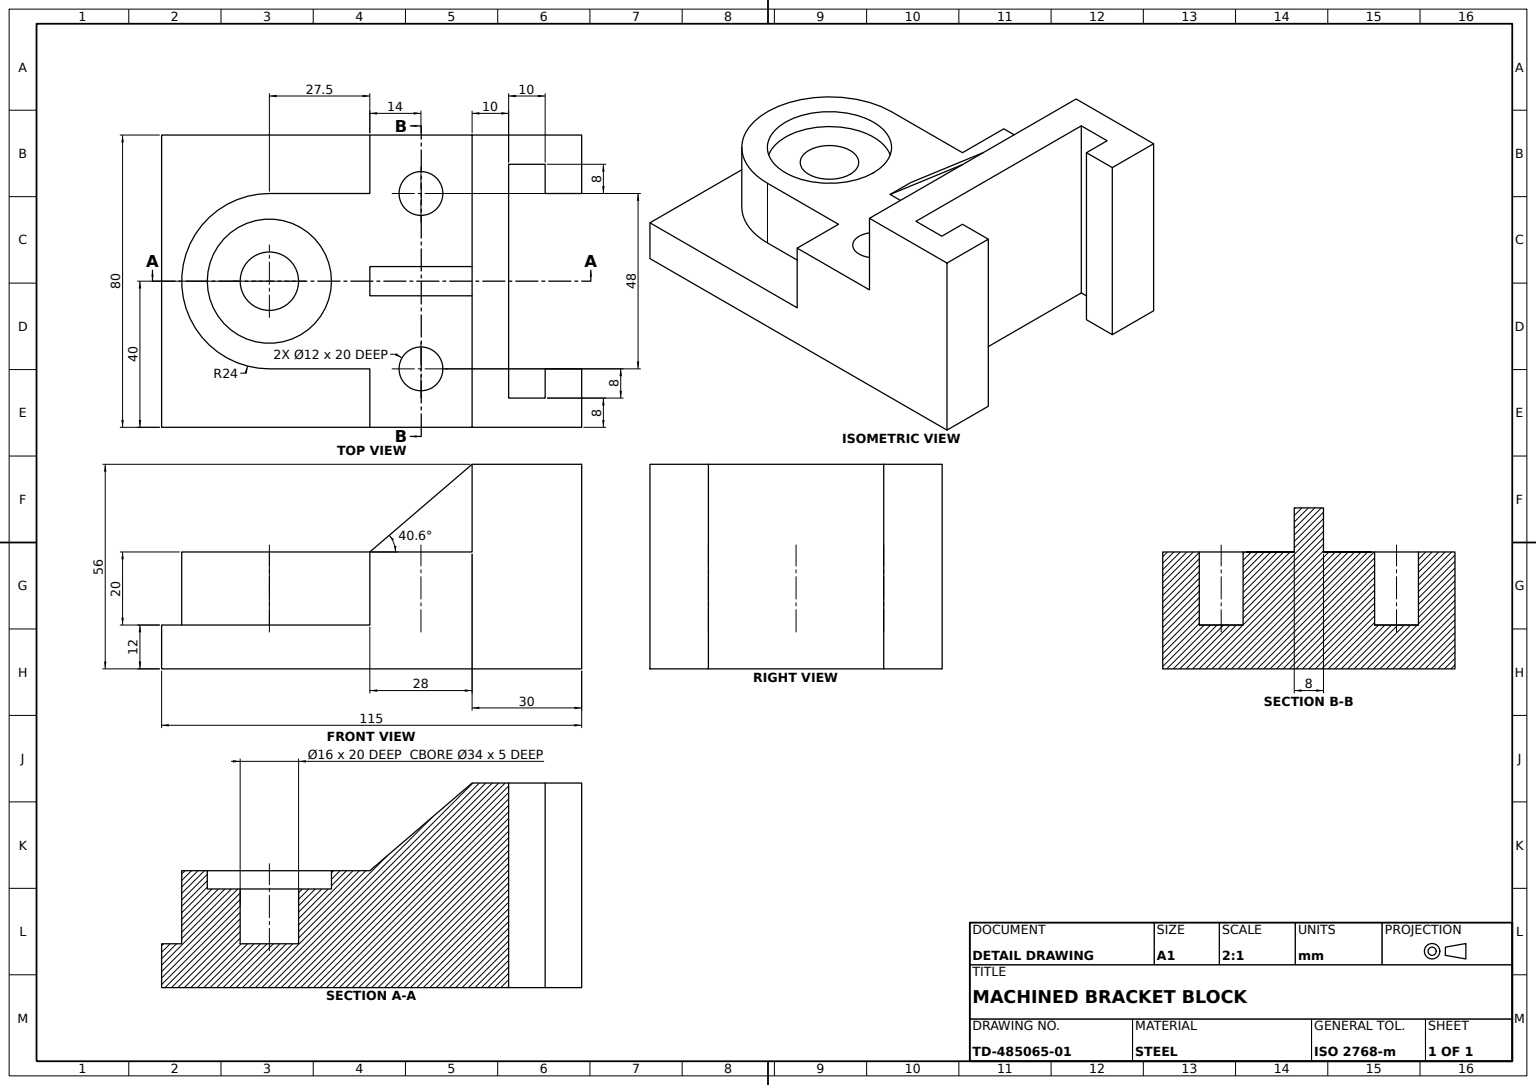
from build123d import *

# Parameters (mm, degrees)
BASE_PLATE_SKETCH_W    = 80
BASE_PLATE_SKETCH_H    = 115
BASE_PLATE_DEPTH       = 12
BACK_WALL_SKETCH_W     = 80
BACK_WALL_SKETCH_H     = 30
BACK_WALL_DEPTH        = 44
WALL_SLOT_CUT_DEPTH    = 90.678592763
BOSS_PAD_SKETCH_R      = 6
BOSS_PAD_DEPTH         = 20
COUNTERBORE_SKETCH_R   = 17
COUNTERBORE_34X5_DEPTH = 5
BORE_SKETCH_R          = 8
BORE_16_DEPTH          = 15
SUPPORT_RIB_8MM_REACH  = 91.679
RIB_SKETCH_WALL_W      = 218.235363356
RIB_SKETCH_WALL_H      = 8


with BuildPart() as part:
    # Base Plate Sketch → Base Plate (new body)
    with BuildSketch(Plane(origin=(0, 0, 0), x_dir=(1, 0, 0), z_dir=(0, 1, 0))):
        Rectangle(BASE_PLATE_SKETCH_W, BASE_PLATE_SKETCH_H)
    extrude(amount=BASE_PLATE_DEPTH)

    # Back Wall Sketch → Back Wall (add)
    with BuildSketch(Plane(origin=(0, 12, 0), x_dir=(1, 0, 0), z_dir=(0, 1, 0))):
        with Locations((0, 42.5)):
            Rectangle(BACK_WALL_SKETCH_W, BACK_WALL_SKETCH_H)
    extrude(amount=BACK_WALL_DEPTH)

    # Wall Slot Sketch → Wall Slot Cut (cut, through all)
    with BuildSketch(Plane(origin=(0, 56, 0), x_dir=(1, 0, 0), z_dir=(0, 1, 0))):
        Polygon((-24, 57.5), (-24, 47.5), (-32, 47.5), (-32, 37.5), (32, 37.5), (32, 47.5), (24, 47.5), (24, 57.5), align=None)
    extrude(amount=-WALL_SLOT_CUT_DEPTH, mode=Mode.SUBTRACT)

    # Boss Pad Sketch → Boss Pad (add)
    with BuildSketch(Plane(origin=(0, 12, 0), x_dir=(1, 0, 0), z_dir=(0, 1, 0))):
        with BuildLine():
            Line((-40, 27.5), (40, 27.5))
            Line((40, 27.5), (40, -0.5))
            Line((40, -0.5), (24, -0.5))
            Line((24, -0.5), (24, -28))
            ThreePointArc((24, -28), (0, -52), (-24, -28))
            Line((-24, -28), (-24, -0.5))
            Line((-24, -0.5), (-40, -0.5))
            Line((-40, -0.5), (-40, 27.5))
        make_face()
        with Locations(Location((-24, 13.5, 0), (0, 0, 270))):
            Circle(BOSS_PAD_SKETCH_R, mode=Mode.SUBTRACT)
        with Locations(Location((24, 13.5, 0), (0, 0, 270))):
            Circle(BOSS_PAD_SKETCH_R, mode=Mode.SUBTRACT)
    extrude(amount=BOSS_PAD_DEPTH)

    # Counterbore Sketch → Counterbore Ø34x5 (cut)
    with BuildSketch(Plane(origin=(0, 32, 0), x_dir=(1, 0, 0), z_dir=(0, 1, 0))):
        with Locations(Location((0, -28, 0), (0, 0, 270))):
            Circle(COUNTERBORE_SKETCH_R)
    extrude(amount=-COUNTERBORE_34X5_DEPTH, mode=Mode.SUBTRACT)

    # Bore Sketch → Bore Ø16 (cut)
    with BuildSketch(Plane(origin=(0, 27, 0), x_dir=(1, 0, 0), z_dir=(0, 1, 0))):
        with Locations(Location((0, -28, 0), (0, 0, 270))):
            Circle(BORE_SKETCH_R)
    extrude(amount=-BORE_16_DEPTH, mode=Mode.SUBTRACT)

    # Rib Sketch wall → Support Rib 8mm (add, up to next)
    with BuildSketch(Plane(origin=(0, 44, -13.5), x_dir=(0, -0.650791373456, 0.759256602365), z_dir=(0, -0.759256602365, -0.650791373456)), mode=Mode.PRIVATE) as support_rib_8mm_sk1:
        Rectangle(RIB_SKETCH_WALL_W, RIB_SKETCH_WALL_H)
    support_rib_8mm_tool1 = extrude(support_rib_8mm_sk1.sketch, amount=SUPPORT_RIB_8MM_REACH, mode=Mode.PRIVATE) - part.part
    add(support_rib_8mm_tool1.solids().sort_by_distance((0, 44, -13.5))[0])


solid = part.part
